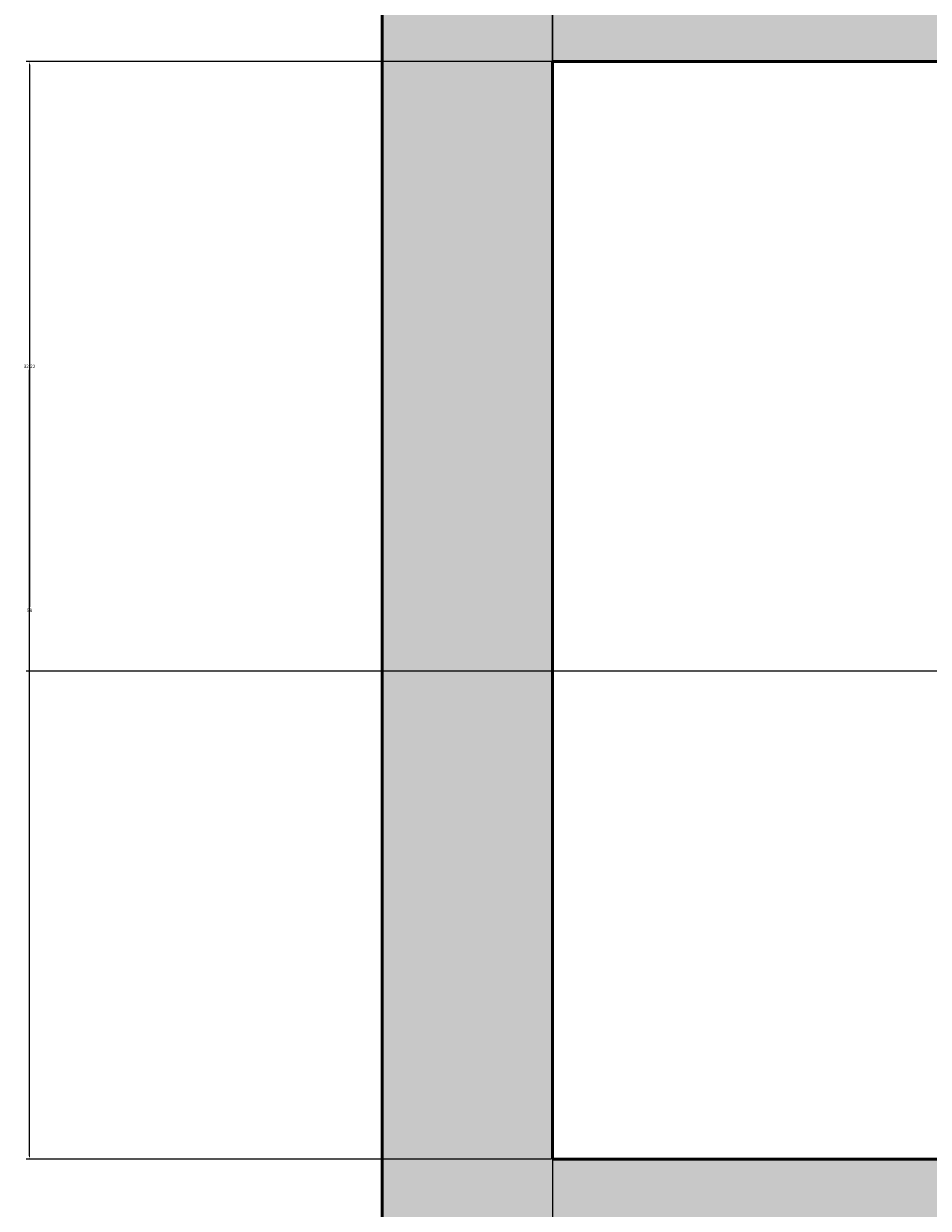
# Model space of a CAD drawing. Units: inches. Extents: x 2231 to 2461, y 2045 to 2455.
# Tile 8 of 95: x 2231 to 2279, y 2122 to 2185. Entities that reach past the tile are written whole.
import ezdxf

# ---------------------------------------------------------------- set-up
doc = ezdxf.new("R2010")
doc.units = ezdxf.units.IN
doc.layers.add('A-ANNO-DIMS', color=2, linetype='Continuous', lineweight=18)
doc.layers.add('A-WALL', color=7, linetype='Continuous', lineweight=50)
doc.layers.add('A-WALL-PATT', color=18, linetype='Continuous', lineweight=13, true_color=0x000000)
doc.styles.get("Standard").update_dxf_attribs({"font": 'arial.ttf'})
doc.dimstyles.get("Standard").update_dxf_attribs({"dimtxt": 0.18, "dimasz": 0.18, "dimexe": 0.18, "dimexo": 0.0625, "dimgap": 0.09, "dimtad": 0, "dimtih": 1, "dimtoh": 1, "dimdec": 4, "dimzin": 0, "dimdsep": 46, "dimtxsty": 'Standard', "dimcen": 0.09, "dimadec": 0, "dimazin": 0, "dimtfac": 1, "dimtdec": 4, "dimtofl": 0, "dimtmove": 0, "dimatfit": 3, "dimfxl": 1, "dimtolj": 1, "dimtzin": 0, "dimarcsym": 0})

# ---------------------------------------------------------------- blocks, each defined once
blk = doc.blocks.new('*D47')
at = {"layer": 'A-ANNO-DIMS', "color": 0, "lineweight": -2, "transparency": 16777216}
for p, q in [((2258.794, 2182.895), (2258.794, 2454.645)), ((2294.794, 2182.895), (2294.794, 2454.645)), ((2258.974, 2454.465), (2276.575, 2454.465)), ((2294.614, 2454.465), (2277.012, 2454.465))]:
    blk.add_line(p, q, dxfattribs=at)
at = {"layer": 'A-ANNO-DIMS', "color": 0, "transparency": 16777216}
for points in [[(2258.974, 2454.495), (2258.974, 2454.435), (2258.794, 2454.465)], [(2294.614, 2454.495), (2294.614, 2454.435), (2294.794, 2454.465)]]:
    blk.add_solid(points, dxfattribs=at)
at = {"layer": 'Defpoints', "color": 0, "transparency": 16777216}
for p in [(2294.794, 2454.465), (2258.794, 2182.833), (2294.794, 2182.833)]:
    blk.add_point(p, dxfattribs=at)
at = {"layer": 'A-ANNO-DIMS', "color": 0, "transparency": 16777216, "insert": (2276.794, 2454.465), "char_height": 0.18, "attachment_point": 5}
blk.add_mtext('\\A1;36', dxfattribs=at)
blk = doc.blocks.new('*D48')
at = {"layer": 'A-ANNO-DIMS', "color": 0, "lineweight": -2, "transparency": 16777216}
for p, q in [((2258.731, 2182.833), (2230.981, 2182.833)), ((2231.161, 2182.653), (2231.161, 2154.015)), ((2231.161, 2125.013), (2231.161, 2153.651)), ((2258.731, 2124.833), (2230.981, 2124.833))]:
    blk.add_line(p, q, dxfattribs=at)
at = {"layer": 'A-ANNO-DIMS', "color": 0, "transparency": 16777216}
for points in [[(2231.131, 2182.653), (2231.191, 2182.653), (2231.161, 2182.833)], [(2231.131, 2125.013), (2231.191, 2125.013), (2231.161, 2124.833)]]:
    blk.add_solid(points, dxfattribs=at)
at = {"layer": 'Defpoints', "color": 0, "transparency": 16777216}
for p in [(2231.161, 2182.833), (2258.794, 2182.833), (2258.794, 2124.833)]:
    blk.add_point(p, dxfattribs=at)
at = {"layer": 'A-ANNO-DIMS', "color": 0, "transparency": 16777216, "insert": (2231.161, 2153.833), "char_height": 0.18, "attachment_point": 5}
blk.add_mtext('\\A1;58', dxfattribs=at)
blk = doc.blocks.new('*D51')
at = {"layer": 'A-ANNO-DIMS', "color": 0, "lineweight": -2, "transparency": 16777216}
for p, q in [((2258.794, 2306.77), (2258.794, 2044.803)), ((2330.794, 2306.77), (2330.794, 2044.803)), ((2258.974, 2044.983), (2294.576, 2044.983)), ((2330.614, 2044.983), (2295.011, 2044.983))]:
    blk.add_line(p, q, dxfattribs=at)
at = {"layer": 'A-ANNO-DIMS', "color": 0, "transparency": 16777216}
for points in [[(2258.974, 2045.013), (2258.974, 2044.953), (2258.794, 2044.983)], [(2330.614, 2045.013), (2330.614, 2044.953), (2330.794, 2044.983)]]:
    blk.add_solid(points, dxfattribs=at)
at = {"layer": 'Defpoints', "color": 0, "transparency": 16777216}
for p in [(2258.794, 2306.833), (2330.794, 2306.833), (2330.794, 2044.983)]:
    blk.add_point(p, dxfattribs=at)
at = {"layer": 'A-ANNO-DIMS', "color": 0, "transparency": 16777216, "insert": (2294.794, 2044.983), "char_height": 0.18, "attachment_point": 5}
blk.add_mtext('\\A1;72', dxfattribs=at)
blk = doc.blocks.new('*D60')
at = {"layer": 'A-ANNO-DIMS', "color": 0, "lineweight": -2, "transparency": 16777216}
for p, q in [((2432.731, 2182.833), (2230.981, 2182.833)), ((2231.161, 2182.653), (2231.161, 2166.906)), ((2231.161, 2150.795), (2231.161, 2166.542)), ((2432.731, 2150.615), (2230.981, 2150.615))]:
    blk.add_line(p, q, dxfattribs=at)
at = {"layer": 'A-ANNO-DIMS', "color": 0, "transparency": 16777216}
for points in [[(2231.131, 2182.653), (2231.191, 2182.653), (2231.161, 2182.833)], [(2231.131, 2150.795), (2231.191, 2150.795), (2231.161, 2150.615)]]:
    blk.add_solid(points, dxfattribs=at)
at = {"layer": 'Defpoints', "color": 0, "transparency": 16777216}
for p in [(2231.161, 2182.833), (2432.794, 2182.833), (2432.794, 2150.615)]:
    blk.add_point(p, dxfattribs=at)
at = {"layer": 'A-ANNO-DIMS', "color": 0, "transparency": 16777216, "insert": (2231.161, 2166.724), "char_height": 0.18, "attachment_point": 5}
blk.add_mtext('\\A1;32.22', dxfattribs=at)

msp = doc.modelspace()

# ---------------------------------------------------------------- hatches: boundary and pattern name
at = {"layer": 'A-WALL-PATT'}
h = msp.add_hatch(color=256, dxfattribs=at)
h.dxf.hatch_style = 1
h.paths.add_polyline_path([(2441.7935, 2269.1535), (2432.7935, 2269.1535), (2432.7935, 2186.8328), (2396.7935, 2186.8328), (2396.7935, 2286.8328), (2394.7935, 2286.8328), (2394.7935, 2186.8328), (2334.7935, 2186.8328), (2334.7935, 2182.8328), (2432.7935, 2182.8328), (2432.7935, 2072.8328), (2416.6639, 2072.8328), (2416.6639, 2063.8328), (2441.7935, 2063.8328)])
h.paths.add_polyline_path([(2368.6639, 2072.8328), (2367.04, 2072.8328), (2330.7942, 2072.8328), (2330.7397, 2063.8328), (2368.6639, 2063.8328)])
h.paths.add_polyline_path([(2300.7392, 2068.3328), (2300.7392, 2072.8328), (2298.7935, 2072.8328), (2294.7935, 2072.8328), (2258.7935, 2072.8328), (2258.7935, 2120.8328), (2294.7935, 2120.8328), (2298.7935, 2120.8328), (2298.7935, 2128.8328), (2294.7935, 2128.8328), (2294.7935, 2124.8328), (2258.7935, 2124.8328), (2258.7935, 2182.8328), (2294.7935, 2182.8328), (2294.7935, 2174.8328), (2298.7935, 2174.8328), (2298.7935, 2182.8328), (2304.7935, 2182.8328), (2304.7935, 2186.8328), (2258.7935, 2186.8328), (2258.7935, 2221.999), (2249.7935, 2221.999), (2249.7935, 2063.8328), (2300.7392, 2063.8328)])
h.paths.add_polyline_path([(2391.9338, 2435.8328), (2333.82, 2435.8328), (2333.82, 2426.8328), (2368.7935, 2426.8328), (2368.7935, 2374.9508), (2368.7935, 2370.8328), (2372.3935, 2370.8328), (2372.7935, 2370.8328), (2372.7935, 2426.8328), (2391.9338, 2426.8328)])
h.paths.add_polyline_path([(2441.7935, 2435.8328), (2415.9338, 2435.8328), (2415.9338, 2426.8328), (2432.7935, 2426.8328), (2432.7935, 2334.8328), (2372.7935, 2334.8328), (2372.7935, 2346.8328), (2368.7935, 2346.8328), (2368.7935, 2306.8328), (2360.7935, 2306.8328), (2360.7935, 2302.8328), (2368.7935, 2302.8328), (2372.7935, 2302.8328), (2372.7935, 2330.8328), (2432.7935, 2330.8328), (2432.7935, 2317.1535), (2441.7935, 2317.1535)])
h.paths.add_polyline_path([(2285.82, 2435.8328), (2249.7935, 2435.8328), (2249.7935, 2269.999), (2258.7935, 2269.999), (2258.7935, 2302.8328), (2318.8168, 2302.8328), (2330.7935, 2302.8328), (2330.7935, 2306.8328), (2258.7935, 2306.8328), (2258.7935, 2426.8328), (2285.82, 2426.8328)])

# ---------------------------------------------------------------- linework, layer by layer
at = {"layer": 'A-WALL'}
for p, q in [((2258.7935, 2182.8328), (2294.7935, 2182.8328)), ((2258.7935, 2124.8328), (2258.7935, 2182.8328)), ((2258.7935, 2124.8328), (2294.7935, 2124.8328))]:
    msp.add_line(p, q, dxfattribs=at)
msp.add_lwpolyline([(2300.7392, 2063.8328), (2249.7935, 2063.8328), (2249.7935, 2435.8328), (2441.7935, 2435.8328), (2441.7935, 2063.8328), (2330.7397, 2063.8328)], dxfattribs=at)

# ---------------------------------------------------------------- dimensions: what is measured, and where the dimension line sits
at = {"layer": 'A-ANNO-DIMS'}
for base, p1, p2, picture, middle in [((2294.7935, 2454.4653), (2258.7935, 2182.8328), (2294.7935, 2182.8328), '*D47', (2276.7935, 2454.4653)), ((2330.7935, 2044.9825), (2258.7935, 2306.8328), (2330.7935, 2306.8328), '*D51', (2294.7935, 2044.9825))]:
    dim = msp.add_linear_dim(base=base, p1=p1, p2=p2, dimstyle='Standard', override={"dimdec": 0, "dimlfac": 1, "dimrnd": 0, "dimzin": 0, "dimdsep": 46, "dimlunit": 2}, dxfattribs=at)
    dim.commit()
    dim.dimension.update_dxf_attribs({"geometry": picture, "text_midpoint": middle})
for p1, p2, override, picture, middle in [((2432.7935, 2150.6145), (2432.7935, 2182.8328), {"dimdec": 2, "dimlfac": 1, "dimrnd": 0, "dimzin": 0, "dimdsep": 46, "dimlunit": 2}, '*D60', (2231.161, 2166.7237)), ((2258.7935, 2124.8328), (2258.7935, 2182.8328), {"dimdec": 0, "dimlfac": 1, "dimrnd": 0, "dimzin": 0, "dimdsep": 46, "dimlunit": 2}, '*D48', (2231.161, 2153.8328))]:
    dim = msp.add_linear_dim(base=(2231.161, 2182.8328), p1=p1, p2=p2, angle=90, dimstyle='Standard', override=override, dxfattribs=at)
    dim.commit()
    dim.dimension.update_dxf_attribs({"geometry": picture, "text_midpoint": middle})

doc.saveas('drawing.dxf')
